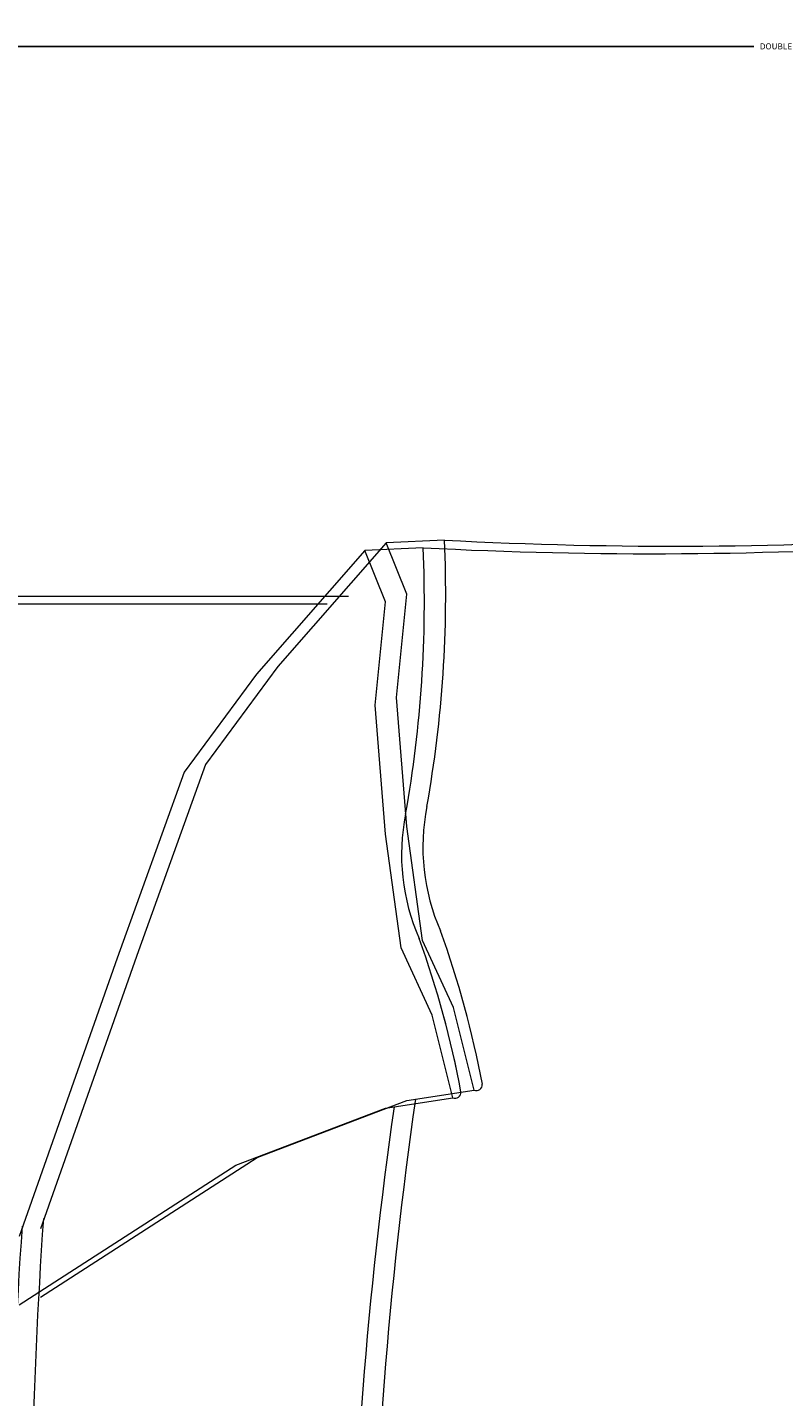
# Model space of a CAD drawing. Units: inches. Extents: x 963 to 2075, y 289 to 2657.
# Tile 41 of 98: x 1533 to 1555, y 1615 to 1656. Entities that reach past the tile are written whole.
import ezdxf

# ---------------------------------------------------------------- set-up
doc = ezdxf.new("R2010")
doc.units = ezdxf.units.IN
doc.layers.add('A-ANNO-DIMS', color=2, linetype='Continuous', lineweight=18)
doc.layers.add('A-FURN', color=8, linetype='Continuous', lineweight=18)
doc.styles.get("Standard").update_dxf_attribs({"font": 'arial.ttf'})
doc.dimstyles.get("Standard").update_dxf_attribs({"dimtxt": 0.18, "dimasz": 0.18, "dimexe": 0.18, "dimexo": 0.0625, "dimgap": 0.09, "dimtad": 0, "dimtih": 1, "dimtoh": 1, "dimdec": 4, "dimzin": 0, "dimdsep": 46, "dimtxsty": 'Standard', "dimcen": 0.09, "dimadec": 0, "dimazin": 0, "dimtfac": 1, "dimtdec": 4, "dimtofl": 0, "dimtmove": 0, "dimatfit": 3, "dimfxl": 1, "dimtolj": 1, "dimtzin": 0, "dimarcsym": 0})

# ---------------------------------------------------------------- blocks, each defined once
blk = doc.blocks.new('BED-DOUBLE')
for p, q in [((1236.849, 2423.736), (1230.356, 2419.546)), ((1236.849, 2423.735), (1230.356, 2419.545)), ((1237.488, 2423.964), (1230.995, 2419.774)), ((1237.488, 2423.964), (1230.995, 2419.774)), ((1233.916, 2413.351), (1236.849, 2421.689)), ((1233.916, 2413.35), (1236.849, 2421.688)), ((1234.555, 2413.579), (1237.488, 2421.917)), ((1234.555, 2413.579), (1237.488, 2421.917)), ((1230.356, 2419.546), (1225.867, 2417.842)), ((1230.356, 2419.545), (1225.867, 2417.842)), ((1230.995, 2419.774), (1226.507, 2418.07)), ((1230.995, 2419.774), (1226.507, 2418.07)), ((1226.507, 2418.07), (1224.495, 2417.76)), ((1226.507, 2418.07), (1224.495, 2417.761)), ((1225.867, 2417.842), (1223.855, 2417.532)), ((1225.867, 2417.842), (1223.855, 2417.532)), ((1223.855, 2417.532), (1224.474, 2415.054)), ((1223.855, 2417.532), (1224.474, 2415.054)), ((1224.495, 2417.761), (1225.114, 2415.283)), ((1224.495, 2417.76), (1225.114, 2415.282)), ((1224.474, 2415.054), (1225.403, 2413.041)), ((1224.474, 2415.054), (1225.403, 2413.041)), ((1225.114, 2415.283), (1226.042, 2413.269)), ((1225.114, 2415.282), (1226.042, 2413.269)), ((1232.543, 2408.003), (1234.555, 2413.579)), ((1232.543, 2408.004), (1234.555, 2413.579)), ((1225.403, 2413.041), (1225.867, 2409.633)), ((1225.403, 2413.041), (1225.867, 2409.634)), ((1226.042, 2413.269), (1226.507, 2409.862)), ((1226.042, 2413.269), (1226.507, 2409.862)), ((1231.904, 2407.775), (1233.916, 2413.351)), ((1231.904, 2407.775), (1233.916, 2413.35)), ((1226.507, 2409.862), (1226.816, 2405.99)), ((1226.507, 2409.862), (1226.816, 2405.99)), ((1225.867, 2409.634), (1226.177, 2405.762)), ((1225.867, 2409.633), (1226.177, 2405.762)), ((1229.737, 2404.832), (1231.904, 2407.775)), ((1229.737, 2404.833), (1231.904, 2407.775)), ((1230.376, 2405.061), (1232.543, 2408.004)), ((1230.376, 2405.061), (1232.543, 2408.003)), ((1226.177, 2405.762), (1225.867, 2402.664)), ((1226.177, 2405.762), (1225.867, 2402.664)), ((1226.816, 2405.99), (1226.507, 2402.892)), ((1226.816, 2405.99), (1226.507, 2402.893)), ((1226.487, 2401.127), (1229.737, 2404.833)), ((1226.487, 2401.127), (1229.737, 2404.832)), ((1227.126, 2401.355), (1230.376, 2405.061)), ((1227.126, 2401.356), (1230.376, 2405.061)), ((1226.507, 2402.893), (1227.126, 2401.356)), ((1226.507, 2402.892), (1227.126, 2401.355)), ((1254.232, 2402.729), (1227.623, 2402.729)), ((1254.232, 2402.729), (1227.623, 2402.729)), ((1254.872, 2402.958), (1228.262, 2402.958)), ((1254.872, 2402.958), (1228.262, 2402.958)), ((1225.867, 2402.664), (1226.487, 2401.127)), ((1225.867, 2402.664), (1226.487, 2401.127)), ((1224.742, 2401.048), (1226.487, 2401.127, 3.871)), ((1224.742, 2401.048), (1226.487, 2401.127, 3.871)), ((1225.381, 2401.276), (1227.126, 2401.356, 3.871)), ((1225.381, 2401.276), (1227.126, 2401.355, 3.871))]:
    blk.add_line(p, q)
for centre, radius, start, end in [((1098.555, 2436.467), 129.02, 351.78449, 6.90062), ((1098.555, 2436.468), 129.02, 351.78449, 6.90062), ((1072.18, 2432.636), 164.969, 356.08655, 6.78213), ((1072.18, 2432.636), 164.969, 356.08655, 6.78213), ((1072.819, 2432.864), 164.969, 356.08655, 6.78213), ((1072.819, 2432.864), 164.969, 356.08655, 6.78213), ((1097.916, 2436.239), 129.02, 351.78449, 6.90062), ((1097.916, 2436.239), 129.02, 351.78449, 6.90062), ((1223.793, 2417.358), 0.185, 70.2464, 181.1377), ((1223.793, 2417.359), 0.185, 70.2464, 181.1377), ((1224.432, 2417.587), 0.185, 70.2464, 181.1377), ((1224.432, 2417.587), 0.185, 70.2464, 181.1377), ((1253.39, 2423.069), 29.654, 190.6617, 199.8806), ((1253.39, 2423.07), 29.654, 190.6617, 199.8806), ((1252.75, 2422.841), 29.654, 190.6617, 199.8806), ((1252.75, 2422.841), 29.654, 190.6617, 199.8806), ((1219.805, 2410.479), 6.224, 348.6608, 23.7384), ((1219.805, 2410.48), 6.224, 348.6608, 23.7384), ((1219.166, 2410.251), 6.224, 348.6608, 23.7384), ((1219.166, 2410.251), 6.224, 348.6608, 23.7384), ((1260.889, 2402.668), 36.183, 169.8763, 182.5657), ((1260.889, 2402.667), 36.183, 169.8763, 182.5657), ((1261.528, 2402.896), 36.183, 169.8763, 182.5657), ((1261.528, 2402.896), 36.183, 169.8763, 182.5657), ((1217.917, 2271.729), 129.499, 86.97912, 93.83645), ((1217.917, 2271.729), 129.499, 86.97912, 93.83645), ((1218.557, 2271.957), 129.499, 86.97912, 93.83645), ((1218.557, 2271.957), 129.499, 86.97912, 93.83645)]:
    blk.add_arc(centre, radius, start, end)
blk = doc.blocks.new('*D14')
at = {"layer": 'A-ANNO-DIMS', "color": 0, "lineweight": -2, "transparency": 16777216}
for p, q in [((1515.065, 1643.568), (1515.065, 1655.918)), ((1515.245, 1655.738), (1554.47, 1655.738)), ((1596.434, 1655.738), (1557.208, 1655.738)), ((1596.614, 1643.568), (1596.614, 1655.918))]:
    blk.add_line(p, q, dxfattribs=at)
at = {"layer": 'A-ANNO-DIMS', "color": 0, "transparency": 16777216}
for points in [[(1515.245, 1655.768), (1515.245, 1655.708), (1515.065, 1655.738)], [(1596.434, 1655.768), (1596.434, 1655.708), (1596.614, 1655.738)]]:
    blk.add_solid(points, dxfattribs=at)
at = {"layer": 'Defpoints', "color": 0, "transparency": 16777216}
for p in [(1515.065, 1655.738), (1515.065, 1643.505), (1596.614, 1643.505)]:
    blk.add_point(p, dxfattribs=at)
at = {"layer": 'A-ANNO-DIMS', "color": 0, "transparency": 16777216, "insert": (1555.839, 1655.738), "char_height": 0.18, "attachment_point": 5}
blk.add_mtext('\\A1;DOUBLE BED 82 TYP.', dxfattribs=at)

msp = doc.modelspace()

# ---------------------------------------------------------------- block references
at = {"layer": 'A-FURN', "rotation": 180}
msp.add_blockref('BED-DOUBLE', (2769.937, 4041.99), dxfattribs=at)

# ---------------------------------------------------------------- dimensions: what is measured, and where the dimension line sits
at = {"layer": 'A-ANNO-DIMS'}
dim = msp.add_linear_dim(base=(1515.065, 1655.738), p1=(1596.614, 1643.505), p2=(1515.065, 1643.505), angle=180, text='DOUBLE BED <> TYP.', dimstyle='Standard', override={"dimdec": 0, "dimlfac": 1, "dimrnd": 0, "dimzin": 0, "dimdsep": 46, "dimlunit": 2}, dxfattribs=at)
dim.commit()
dim.dimension.update_dxf_attribs({"geometry": '*D14', "text_midpoint": (1555.839, 1655.738)})

doc.saveas('drawing.dxf')
